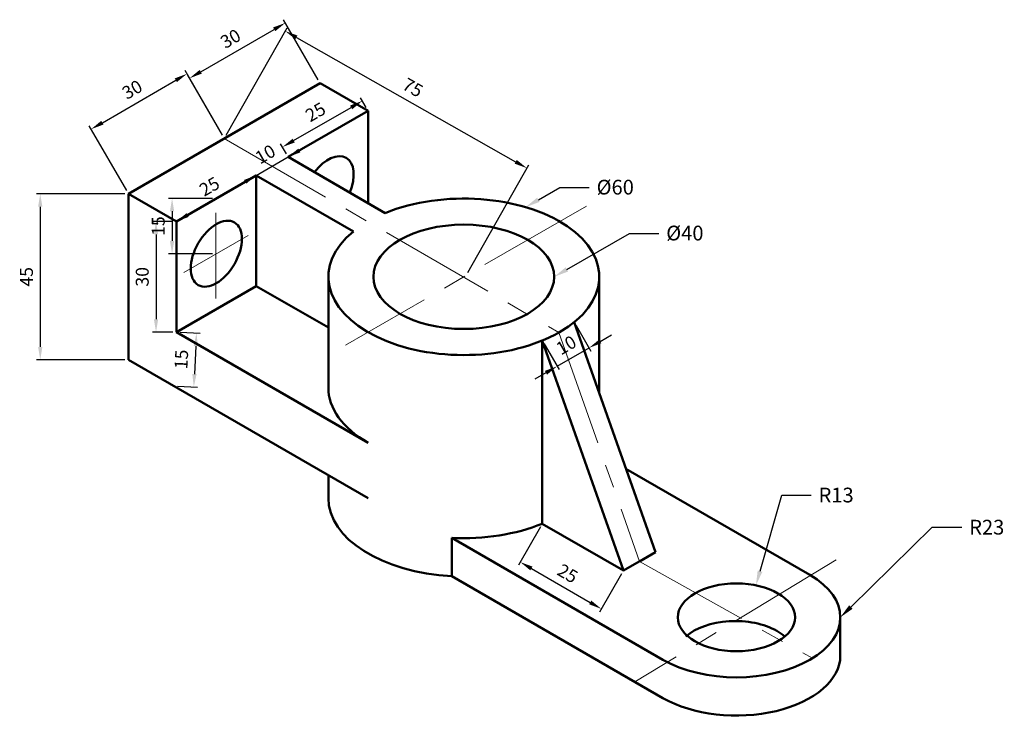
# Model space of a CAD drawing. Units: millimetres. Extents: x 1298 to 1565, y 742 to 932.
import ezdxf
from ezdxf import colors
from ezdxf.entities.mleader import LeaderData, LeaderLine
from ezdxf.math import Vec2, Vec3

# ---------------------------------------------------------------- set-up
doc = ezdxf.new("R2010")
doc.units = ezdxf.units.MM
doc.linetypes.add('CENTER', pattern=[50.8, 31.75, -6.35, 6.35, -6.35])
for name, color, linetype, lineweight in [('M-CNTR', 4, 'CENTER', 18), ('M-DIMS', 3, 'Continuous', 25), ('M-OUTL', 7, 'Continuous', 50), ('M-TEXT', 3, 'Continuous', 25)]:
    doc.layers.add(name, color=color, linetype=linetype, lineweight=lineweight)
doc.styles.get("Standard").update_dxf_attribs({"font": 'arial.ttf'})
doc.dimstyles.new('AM_ISO$0', dxfattribs={"dimtxt": 3.5, "dimasz": 3.5, "dimexe": 1, "dimexo": 1, "dimgap": 1.5, "dimtad": 1, "dimdsep": 46, "dimtxsty": 'Standard', "dimcen": 0, "dimclrd": 256, "dimclre": 256, "dimclrt": 2, "dimadec": 0, "dimazin": 2, "dimtp": 0.1, "dimtm": 0.1, "dimtfac": 0.71, "dimtdec": 3, "dimtmove": 0, "dimatfit": 3, "dimfxl": 1, "dimlwd": -1, "dimlwe": -1, "dimarcsym": 1})

# ---------------------------------------------------------------- blocks, each defined once
blk = doc.blocks.new('*D3')
at = {"layer": 'Defpoints', "color": 0, "transparency": 16777216}
for p in [(1353.34, 899.84), (1435.39, 891.8), (1418.88, 862.68)]:
    blk.add_point(p, dxfattribs=at)
at = {"layer": 'M-DIMS', "color": 0, "linetype": 'ByBlock', "transparency": 16777216}
for p, q in [((1353.83, 900.71), (1370.34, 929.83)), ((1372.89, 927.24), (1432.34, 893.53)), ((1419.37, 863.55), (1435.88, 892.67))]:
    blk.add_line(p, q, dxfattribs=at)
at = {"layer": 'M-DIMS', "color": 0, "transparency": 16777216}
for points in [[(1373.18, 927.74), (1372.61, 926.73), (1369.85, 928.96)], [(1432.63, 894.04), (1432.06, 893.02), (1435.39, 891.8)]]:
    blk.add_solid(points, dxfattribs=at)
at = {"layer": 'M-DIMS', "color": 0, "transparency": 16777216, "insert": (1404.24, 913.24), "char_height": 3.5, "attachment_point": 5, "rotation": 330.4463}
blk.add_mtext('75', dxfattribs=at)
blk = doc.blocks.new('*D4')
at = {"layer": 'Defpoints', "color": 0, "transparency": 16777216}
for p in [(1327.36, 884.84), (1303.42, 839.84), (1327.36, 839.84)]:
    blk.add_point(p, dxfattribs=at)
at = {"layer": 'M-DIMS', "color": 0, "linetype": 'ByBlock', "transparency": 16777216}
for p, q in [((1326.36, 884.84), (1302.42, 884.84)), ((1303.42, 881.34), (1303.42, 843.34)), ((1326.36, 839.84), (1302.42, 839.84))]:
    blk.add_line(p, q, dxfattribs=at)
at = {"layer": 'M-DIMS', "color": 0, "transparency": 16777216}
for points in [[(1302.84, 881.34), (1304.01, 881.34), (1303.42, 884.84)], [(1302.84, 843.34), (1304.01, 843.34), (1303.42, 839.84)]]:
    blk.add_solid(points, dxfattribs=at)
at = {"layer": 'M-DIMS', "color": 0, "transparency": 16777216, "insert": (1300.14, 862.34), "char_height": 3.5, "attachment_point": 5, "rotation": 90}
blk.add_mtext('45', dxfattribs=at)
blk = doc.blocks.new('*D5')
at = {"layer": 'Defpoints', "color": 0, "transparency": 16777216}
for p in [(1343.21, 917.37), (1353.34, 899.84), (1327.36, 884.84)]:
    blk.add_point(p, dxfattribs=at)
at = {"layer": 'M-DIMS', "color": 0, "linetype": 'ByBlock', "transparency": 16777216}
for p, q in [((1352.84, 900.71), (1342.71, 918.24)), ((1320.26, 904.12), (1340.18, 915.62)), ((1326.86, 885.71), (1316.73, 903.24))]:
    blk.add_line(p, q, dxfattribs=at)
at = {"layer": 'M-DIMS', "color": 0, "transparency": 16777216}
for points in [[(1339.89, 916.13), (1340.47, 915.12), (1343.21, 917.37)], [(1319.97, 904.63), (1320.56, 903.62), (1317.23, 902.37)]]:
    blk.add_solid(points, dxfattribs=at)
at = {"layer": 'M-DIMS', "color": 0, "transparency": 16777216, "insert": (1328.58, 912.72), "char_height": 3.5, "attachment_point": 5, "rotation": 30}
blk.add_mtext('30', dxfattribs=at)
blk = doc.blocks.new('*D6')
at = {"layer": 'Defpoints', "color": 0, "transparency": 16777216}
for p in [(1369.89, 931.17), (1379.32, 914.84), (1353.34, 899.84)]:
    blk.add_point(p, dxfattribs=at)
at = {"layer": 'M-DIMS', "color": 0, "linetype": 'ByBlock', "transparency": 16777216}
for p, q in [((1378.82, 915.71), (1369.39, 932.04)), ((1346.94, 917.92), (1366.86, 929.42)), ((1352.84, 900.71), (1343.41, 917.04))]:
    blk.add_line(p, q, dxfattribs=at)
at = {"layer": 'M-DIMS', "color": 0, "transparency": 16777216}
for points in [[(1366.56, 929.93), (1367.15, 928.92), (1369.89, 931.17)], [(1346.65, 918.43), (1347.23, 917.42), (1343.91, 916.17)]]:
    blk.add_solid(points, dxfattribs=at)
at = {"layer": 'M-DIMS', "color": 0, "transparency": 16777216, "insert": (1355.25, 926.52), "char_height": 3.5, "attachment_point": 5, "rotation": 30}
blk.add_mtext('30', dxfattribs=at)
blk = doc.blocks.new('*D7')
at = {"layer": 'Defpoints', "color": 0, "transparency": 16777216}
for p in [(1370.66, 894.84), (1370.66, 894.84), (1362, 889.84)]:
    blk.add_point(p, dxfattribs=at)
at = {"layer": 'M-DIMS', "color": 0, "linetype": 'ByBlock', "transparency": 16777216}
for p, q in [((1373.69, 896.59), (1376.72, 898.34)), ((1362, 889.84), (1370.66, 894.84)), ((1358.97, 888.09), (1355.93, 886.34))]:
    blk.add_line(p, q, dxfattribs=at)
at = {"layer": 'M-DIMS', "color": 0, "transparency": 16777216}
for points in [[(1373.4, 897.09), (1373.98, 896.08), (1370.66, 894.84)], [(1358.67, 888.59), (1359.26, 887.58), (1362, 889.84)]]:
    blk.add_solid(points, dxfattribs=at)
at = {"layer": 'M-DIMS', "color": 0, "transparency": 16777216, "insert": (1364.68, 895.19), "char_height": 3.5, "attachment_point": 5, "rotation": 30}
blk.add_mtext('10', dxfattribs=at)
blk = doc.blocks.new('*D8')
at = {"layer": 'Defpoints', "color": 0, "transparency": 16777216}
for p in [(1362, 889.84), (1362, 889.84), (1340.35, 877.34)]:
    blk.add_point(p, dxfattribs=at)
at = {"layer": 'M-DIMS', "color": 0, "linetype": 'ByBlock', "transparency": 16777216}
blk.add_line((1343.38, 879.09), (1358.97, 888.09), dxfattribs=at)
at = {"layer": 'M-DIMS', "color": 0, "transparency": 16777216}
for points in [[(1358.67, 888.59), (1359.26, 887.58), (1362, 889.84)], [(1343.09, 879.59), (1343.67, 878.58), (1340.35, 877.34)]]:
    blk.add_solid(points, dxfattribs=at)
at = {"layer": 'M-DIMS', "color": 0, "transparency": 16777216, "insert": (1349.53, 886.44), "char_height": 3.5, "attachment_point": 5, "rotation": 30}
blk.add_mtext('25', dxfattribs=at)
blk = doc.blocks.new('*D9')
at = {"layer": 'Defpoints', "color": 0, "transparency": 16777216}
for p in [(1390.76, 910.02), (1392.31, 907.34), (1370.66, 894.84)]:
    blk.add_point(p, dxfattribs=at)
at = {"layer": 'M-DIMS', "color": 0, "linetype": 'ByBlock', "transparency": 16777216}
for p, q in [((1391.81, 908.21), (1390.26, 910.88)), ((1372.14, 899.27), (1387.73, 908.27)), ((1370.16, 895.71), (1368.61, 898.38))]:
    blk.add_line(p, q, dxfattribs=at)
at = {"layer": 'M-DIMS', "color": 0, "transparency": 16777216}
for points in [[(1387.44, 908.77), (1388.02, 907.76), (1390.76, 910.02)], [(1371.85, 899.77), (1372.43, 898.76), (1369.11, 897.52)]]:
    blk.add_solid(points, dxfattribs=at)
at = {"layer": 'M-DIMS', "color": 0, "transparency": 16777216, "insert": (1378.29, 906.62), "char_height": 3.5, "attachment_point": 5, "rotation": 30}
blk.add_mtext('25', dxfattribs=at)
blk = doc.blocks.new('*D10')
at = {"layer": 'Defpoints', "color": 0, "transparency": 16777216}
for p in [(1340.35, 877.34), (1334.82, 847.34), (1340.35, 847.34)]:
    blk.add_point(p, dxfattribs=at)
at = {"layer": 'M-DIMS', "color": 0, "linetype": 'ByBlock', "transparency": 16777216}
for p, q in [((1339.35, 877.34), (1333.82, 877.34)), ((1334.82, 873.84), (1334.82, 850.84)), ((1339.35, 847.34), (1333.82, 847.34))]:
    blk.add_line(p, q, dxfattribs=at)
at = {"layer": 'M-DIMS', "color": 0, "transparency": 16777216}
for points in [[(1334.23, 873.84), (1335.4, 873.84), (1334.82, 877.34)], [(1334.23, 850.84), (1335.4, 850.84), (1334.82, 847.34)]]:
    blk.add_solid(points, dxfattribs=at)
at = {"layer": 'M-DIMS', "color": 0, "transparency": 16777216, "insert": (1331.53, 862.34), "char_height": 3.5, "attachment_point": 5, "rotation": 90}
blk.add_mtext('30', dxfattribs=at)
blk = doc.blocks.new('*D11')
at = {"layer": 'Defpoints', "color": 0, "transparency": 16777216}
for p in [(1351.17, 883.59), (1339.17, 868.59), (1351.17, 868.59)]:
    blk.add_point(p, dxfattribs=at)
at = {"layer": 'M-DIMS', "color": 0, "linetype": 'ByBlock', "transparency": 16777216}
for p, q in [((1350.17, 883.59), (1338.17, 883.59)), ((1339.17, 880.09), (1339.17, 872.09)), ((1350.17, 868.59), (1338.17, 868.59))]:
    blk.add_line(p, q, dxfattribs=at)
at = {"layer": 'M-DIMS', "color": 0, "transparency": 16777216}
for points in [[(1338.59, 880.09), (1339.75, 880.09), (1339.17, 883.59)], [(1338.59, 872.09), (1339.75, 872.09), (1339.17, 868.59)]]:
    blk.add_solid(points, dxfattribs=at)
at = {"layer": 'M-DIMS', "color": 0, "transparency": 16777216, "insert": (1335.88, 876.09), "char_height": 3.5, "attachment_point": 5, "rotation": 90}
blk.add_mtext('15', dxfattribs=at)
blk = doc.blocks.new('*D12')
at = {"layer": 'Defpoints', "color": 0, "transparency": 16777216}
for p in [(1448.24, 850.05), (1439.58, 845.05), (1452.26, 843.08)]:
    blk.add_point(p, dxfattribs=at)
at = {"layer": 'M-DIMS', "color": 0, "linetype": 'ByBlock', "transparency": 16777216}
for p, q in [((1448.74, 849.18), (1452.76, 842.22)), ((1455.29, 844.83), (1458.32, 846.58)), ((1440.08, 844.18), (1444.1, 837.22)), ((1443.6, 838.08), (1452.26, 843.08)), ((1440.57, 836.33), (1437.54, 834.58))]:
    blk.add_line(p, q, dxfattribs=at)
at = {"layer": 'M-DIMS', "color": 0, "transparency": 16777216}
for points in [[(1455, 845.34), (1455.58, 844.33), (1452.26, 843.08)], [(1440.28, 836.84), (1440.86, 835.83), (1443.6, 838.08)]]:
    blk.add_solid(points, dxfattribs=at)
at = {"layer": 'M-DIMS', "color": 0, "transparency": 16777216, "insert": (1446.28, 843.43), "char_height": 3.5, "attachment_point": 5, "rotation": 30}
blk.add_mtext('10', dxfattribs=at)
blk = doc.blocks.new('*D13')
at = {"layer": 'Defpoints', "color": 0, "transparency": 16777216}
for p in [(1340.35, 847.34), (1339.62, 832.76), (1345.06, 832.49)]:
    blk.add_point(p, dxfattribs=at)
at = {"layer": 'M-DIMS', "color": 0, "linetype": 'ByBlock', "transparency": 16777216}
for p, q in [((1341.34, 847.29), (1346.78, 847.02)), ((1345.61, 843.57), (1345.24, 835.98)), ((1340.62, 832.71), (1346.06, 832.44))]:
    blk.add_line(p, q, dxfattribs=at)
at = {"layer": 'M-DIMS', "color": 0, "transparency": 16777216}
for points in [[(1345.03, 843.6), (1346.19, 843.55), (1345.78, 847.07)], [(1344.65, 836.01), (1345.82, 835.95), (1345.06, 832.49)]]:
    blk.add_solid(points, dxfattribs=at)
at = {"layer": 'M-DIMS', "color": 0, "transparency": 16777216, "insert": (1342.14, 839.94), "char_height": 3.5, "attachment_point": 5, "rotation": 87.1653}
blk.add_mtext('15', dxfattribs=at)
blk = doc.blocks.new('*D14')
at = {"layer": 'Defpoints', "color": 0, "transparency": 16777216}
for p in [(1439.58, 795.42), (1461.59, 782.71), (1455.59, 772.31)]:
    blk.add_point(p, dxfattribs=at)
at = {"layer": 'M-DIMS', "color": 0, "linetype": 'ByBlock', "transparency": 16777216}
for p, q in [((1439.08, 794.55), (1433.08, 784.16)), ((1436.61, 783.27), (1452.56, 774.06)), ((1461.09, 781.84), (1455.09, 771.45))]:
    blk.add_line(p, q, dxfattribs=at)
at = {"layer": 'M-DIMS', "color": 0, "transparency": 16777216}
for points in [[(1436.9, 783.78), (1436.32, 782.77), (1433.58, 785.02)], [(1452.85, 774.57), (1452.27, 773.56), (1455.59, 772.31)]]:
    blk.add_solid(points, dxfattribs=at)
at = {"layer": 'M-DIMS', "color": 0, "transparency": 16777216, "insert": (1446.23, 781.52), "char_height": 3.5, "attachment_point": 5, "rotation": 330}
blk.add_mtext('25', dxfattribs=at)

msp = doc.modelspace()

# ---------------------------------------------------------------- linework, layer by layer
at = {"layer": 'M-CNTR'}
for p, q in [((1353.337, 899.84), (1444.088, 847.236)), ((1451.52, 881.526), (1386.231, 843.831)), ((1351.08, 879.705), (1351.08, 856.429)), ((1359.798, 873.57), (1342.362, 863.503)), ((1444.088, 847.236), (1465.92, 785.207)), ((1519.28, 785.647), (1464.68, 752.555)), ((1465.92, 785.207), (1512.824, 758.934))]:
    msp.add_line(p, q, dxfattribs=at)
at = {"layer": 'M-OUTL'}
for p, q in [((1327.356, 884.84), (1379.317, 914.84)), ((1379.317, 914.84), (1392.308, 907.34)), ((1392.308, 907.34), (1370.657, 894.84)), ((1392.308, 907.34), (1392.308, 882.34)), ((1370.657, 894.84), (1397.001, 879.63)), ((1361.997, 889.84), (1340.346, 877.34)), ((1361.997, 889.84), (1351.171, 883.59)), ((1361.997, 859.84), (1361.997, 889.84)), ((1361.997, 889.84), (1388.341, 874.63)), ((1327.356, 839.84), (1327.356, 884.84)), ((1340.347, 877.34), (1327.356, 884.84)), ((1340.346, 877.34), (1340.346, 847.34)), ((1340.346, 847.34), (1361.997, 859.84)), ((1361.997, 859.84), (1381.546, 848.553)), ((1381.546, 832.34), (1381.546, 862.34)), ((1455.031, 862.34), (1455.031, 830.807)), ((1448.236, 850.049), (1470.25, 787.707)), ((1340.346, 847.34), (1392.308, 817.34)), ((1439.576, 795.417), (1439.576, 845.049)), ((1439.576, 845.049), (1461.59, 782.707)), ((1327.356, 839.84), (1392.308, 802.34)), ((1462.266, 810.316), (1512.137, 781.523)), ((1381.546, 802.34), (1381.546, 808.553)), ((1461.59, 782.707), (1439.576, 795.417)), ((1415.051, 791.576), (1472.3, 758.523)), ((1415.051, 791.576), (1415.051, 781.209)), ((1470.25, 787.707), (1461.59, 782.707)), ((1465.92, 785.207), (1470.25, 787.707)), ((1415.051, 781.209), (1472.3, 748.156)), ((1520.388, 770.023), (1520.388, 759.656))]:
    msp.add_line(p, q, dxfattribs=at)
for centre, major_axis, start_param, end_param in [((1381.482, 886.09), (-4.899, -8.485), 8.0767915, 10.7727645), ((1418.288, 862.34), (-36.742, 0), 5.6652352, 11.6135244), ((1418.288, 832.34), (-36.742, 0), 6.2831853, 7.0685835), ((1418.288, 802.34), (-36.742, 0), 6.2831853, 7.7657466), ((1418.288, 812.707), (-36.742, 0), 7.7657466, 8.4719317), ((1492.219, 770.023), (-28.169, 0), 0.7853982, 3.9269908), ((1491.901, 759.84), (15.922, 0), 0.7853982, 2.5664812), ((1491.901, 759.84), (15.922, 0), 0.5751114, 0.7853982), ((1492.219, 759.656), (-28.169, 0), 0.7853982, 3.1415927)]:
    msp.add_ellipse(centre, major_axis=major_axis, ratio=0.5773503, start_param=start_param, end_param=end_param, dxfattribs=at)
for centre, major_axis in [((1351.171, 868.59), (-4.899, -8.485)), ((1418.288, 862.34), (-24.495, 0)), ((1492.219, 770.023), (-15.922, 0))]:
    msp.add_ellipse(centre, major_axis=major_axis, ratio=0.5773503, dxfattribs=at)

# ---------------------------------------------------------------- dimensions: what is measured, and where the dimension line sits
at = {"layer": 'M-DIMS'}
for p1, p2, distance, override, picture, middle in [((1353.337, 899.84), (1379.317, 914.84), 18.861, {"dimclrd": 0, "dimclre": 0, "dimclrt": 0}, '*D6', (1355.252, 926.521)), ((1327.356, 884.84), (1353.337, 899.84), 20.245, {"dimclrd": 0, "dimclre": 0, "dimclrt": 0}, '*D5', (1328.58, 912.72)), ((1370.657, 894.84), (1392.308, 907.34), 3.093, {"dimclrd": 0, "dimclre": 0, "dimclrt": 0}, '*D9', (1378.292, 906.615)), ((1361.997, 889.84), (1370.657, 894.84), 0, {"dimclrd": 0, "dimclre": 0, "dimclrt": 0}, '*D7', (1364.683, 895.186)), ((1340.346, 877.34), (1361.997, 889.84), 0, {"dimpost": '', "dimclrd": 0, "dimclre": 0, "dimclrt": 0}, '*D8', (1349.528, 886.436)), ((1327.356, 884.84), (1327.356, 839.84), -23.934, {"dimclrd": 0, "dimclre": 0, "dimclrt": 0}, '*D4', (1300.142, 862.34)), ((1351.171, 883.59), (1351.171, 868.59), -12, {"dimpost": '', "dimclrd": 0, "dimclre": 0, "dimclrt": 0}, '*D11', (1335.884, 876.09)), ((1340.346, 877.34), (1340.346, 847.34), -5.531, {"dimclrd": 0, "dimclre": 0, "dimclrt": 0}, '*D10', (1331.527, 862.34)), ((1439.576, 845.049), (1448.236, 850.049), -8.045, {"dimclrd": 0, "dimclre": 0, "dimclrt": 0}, '*D12', (1446.285, 843.429))]:
    dim = msp.add_aligned_dim(p1=p1, p2=p2, distance=distance, dimstyle='AM_ISO$0', override=override, dxfattribs=at)
    dim.commit()
    dim.dimension.update_dxf_attribs({"geometry": picture, "text_midpoint": middle})
for p1, p2, distance, text, picture, middle in [((1353.337, 899.84), (1418.875, 862.678), 33.48, '75', '*D3', (1404.237, 913.236)), ((1340.346, 847.34), (1339.624, 832.756), 5.445, '15', '*D13', (1342.141, 839.941)), ((1439.576, 795.417), (1461.59, 782.707), -12, '25', '*D14', (1446.226, 781.516))]:
    dim = msp.add_aligned_dim(p1=p1, p2=p2, distance=distance, text=text, dimstyle='AM_ISO$0', override={"dimpost": '', "dimclrd": 0, "dimclre": 0, "dimclrt": 0}, dxfattribs=at)
    dim.commit()
    dim.dimension.update_dxf_attribs({"geometry": picture, "text_midpoint": middle})

# ---------------------------------------------------------------- leaders
at = {"layer": 'M-TEXT'}
ml = msp.add_multileader_mtext('Standard', dxfattribs=at)
ml.set_content('{\\C2;%%C60}', color=256)
ml.set_leader_properties()
ml.build(insert=Vec2(0, 0))
ctx = ml.context
ctx.base_point, ctx.plane_origin = Vec3(1452.298, 886.565), Vec3(1435.039, 881.22)
notes = []
notes.append((ctx, [(0, (1, 1, 0), (1444.298, 886.565), (1, 0), 8, [(0, [(1435.039, 881.22)], 0, [])])]))
ctx.mtext.insert, ctx.mtext.flow_direction = Vec3(1454.298, 888.646), 5
ml = msp.add_multileader_mtext('Standard', dxfattribs=at)
ml.set_content('{\\C2;%%C40}', color=256)
ml.set_leader_properties()
ml.build(insert=Vec2(0, 0))
ctx = ml.context
ctx.base_point, ctx.plane_origin = Vec3(1471.18, 874.116), Vec3(1442.783, 862.34)
notes.append((ctx, [(0, (1, 1, 0), (1463.18, 874.116), (1, 0), 8, [(0, [(1442.783, 862.34)], 0, [])])]))
ctx.mtext.insert, ctx.mtext.flow_direction = Vec3(1473.18, 876.196), 5
ml = msp.add_multileader_mtext('Standard', dxfattribs=at)
ml.set_content('{\\C2;R13}', color=256)
ml.set_leader_properties()
ml.build(insert=Vec2(0, 0))
ctx = ml.context
ctx.base_point, ctx.plane_origin = Vec3(1512.496, 803.139), Vec3(1497.51, 778.693)
notes.append((ctx, [(0, (1, 1, 0), (1504.496, 803.139), (1, 0), 8, [(0, [(1497.51, 778.693)], 0, [])])]))
ctx.mtext.insert, ctx.mtext.flow_direction = Vec3(1514.496, 805.174), 5
ml = msp.add_multileader_mtext('Standard', dxfattribs=at)
ml.set_content('{\\C2;R23}', color=256)
ml.set_leader_properties()
ml.build(insert=Vec2(0, 0))
ctx = ml.context
ctx.base_point, ctx.plane_origin = Vec3(1553.339, 794.43), Vec3(1520.388, 770.023)
notes.append((ctx, [(0, (1, 1, 0), (1545.339, 794.43), (1, 0), 8, [(0, [(1520.388, 770.023)], 0, [])])]))
ctx.mtext.insert, ctx.mtext.flow_direction = Vec3(1555.339, 796.466), 5
for ctx, leaders in notes:
    for number, flags, end, landing, length, lines in leaders:
        leader = LeaderData()
        leader.index, (leader.has_last_leader_line, leader.has_dogleg_vector, leader.attachment_direction) = number, flags
        leader.last_leader_point, leader.dogleg_vector, leader.dogleg_length = Vec3(end), Vec3(landing), length
        for number, points, colour, breaks in lines:
            line = LeaderLine()
            line.index, line.vertices, line.color, line.breaks = number, Vec3.list(points), colors.encode_raw_color(colour), breaks
            leader.lines.append(line)
        ctx.leaders.append(leader)

doc.saveas('drawing.dxf')
